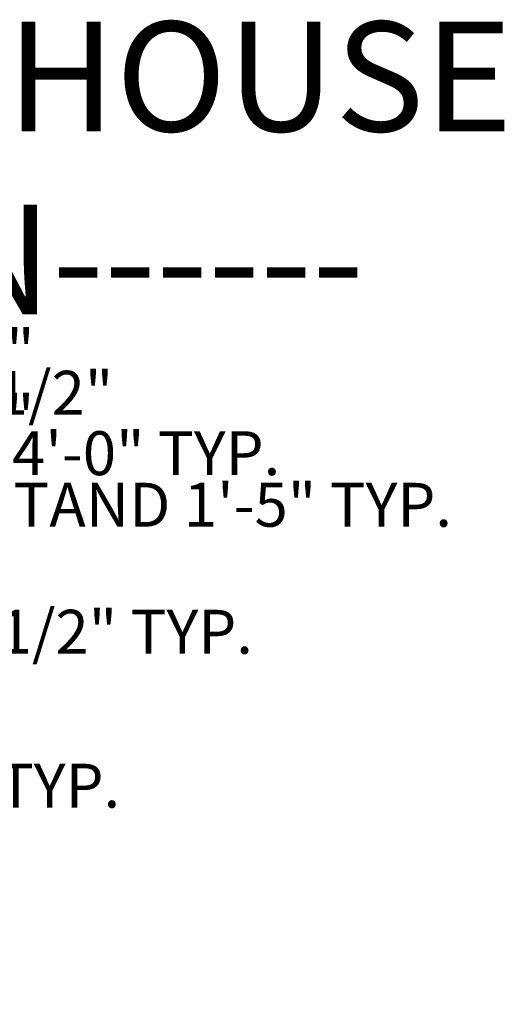
# Model space of a CAD drawing. Units: inches. Extents: x 2838 to 4029, y 1041 to 1915.
# Tile 16 of 16: x 3764 to 4029, y 1377 to 1915. Entities that reach past the tile are written whole.
import ezdxf

# ---------------------------------------------------------------- set-up
doc = ezdxf.new("R2010")
doc.units = ezdxf.units.IN
doc.header["$MEASUREMENT"] = 0
doc.layers.add('A-ANNO-DIMS', color=2, linetype='Continuous', lineweight=18)
doc.layers.add('A-ANNO-TEXT', color=7, linetype='Continuous', lineweight=18)
doc.styles.get("Standard").update_dxf_attribs({"font": 'arial.ttf'})
doc.dimstyles.get("Standard").update_dxf_attribs({"dimtxt": 24, "dimasz": 36, "dimexe": 0.18, "dimexo": 0.0625, "dimgap": 0.09, "dimtad": 0, "dimtih": 1, "dimtoh": 1, "dimdec": 0, "dimzin": 0, "dimdsep": 46, "dimlunit": 3, "dimtxsty": 'Standard', "dimcen": 0.09, "dimadec": 0, "dimazin": 0, "dimtfac": 1, "dimtdec": 0, "dimtofl": 0, "dimtmove": 0, "dimatfit": 3, "dimfxl": 1, "dimtolj": 1, "dimtzin": 0, "dimarcsym": 0})

# ---------------------------------------------------------------- blocks, each defined once
blk = doc.blocks.new('*D27')
at = {"layer": 'A-ANNO-DIMS', "color": 0, "lineweight": -2, "transparency": 16777216}
for p, q in [((3598.68, 1614.31), (3598.68, 1650.31)), ((3598.68, 1650.31), (3634.68, 1650.31)), ((3601.19, 1578.31), (3598.5, 1578.31)), ((3601.19, 1561.16), (3598.5, 1561.16)), ((3598.68, 1525.16), (3598.68, 1489.16))]:
    blk.add_line(p, q, dxfattribs=at)
at = {"layer": 'A-ANNO-DIMS', "color": 0, "transparency": 16777216}
for points in [[(3592.68, 1614.31), (3604.68, 1614.31), (3598.68, 1578.31)], [(3592.68, 1525.16), (3604.68, 1525.16), (3598.68, 1561.16)]]:
    blk.add_solid(points, dxfattribs=at)
at = {"layer": 'Defpoints', "color": 0, "transparency": 16777216}
for p in [(3598.68, 1578.31), (3601.25, 1578.31), (3601.25, 1561.16)]:
    blk.add_point(p, dxfattribs=at)
at = {"layer": 'A-ANNO-DIMS', "color": 0, "transparency": 16777216, "insert": (3820.96, 1650.31), "char_height": 24, "attachment_point": 5}
blk.add_mtext('\\A1;NIGHTSTAND 1\'-5" TYP.', dxfattribs=at)
blk = doc.blocks.new('*D28')
at = {"layer": 'A-ANNO-DIMS', "color": 0, "lineweight": -2, "transparency": 16777216}
for p, q in [((3565.25, 1580.88), (3529.25, 1580.88)), ((3601.25, 1578.37), (3601.25, 1581.06)), ((3617.82, 1578.37), (3617.82, 1581.06)), ((3653.82, 1580.88), (3689.82, 1580.88))]:
    blk.add_line(p, q, dxfattribs=at)
at = {"layer": 'A-ANNO-DIMS', "color": 0, "transparency": 16777216}
for points in [[(3565.25, 1586.88), (3565.25, 1574.88), (3601.25, 1580.88)], [(3653.82, 1586.88), (3653.82, 1574.88), (3617.82, 1580.88)]]:
    blk.add_solid(points, dxfattribs=at)
at = {"layer": 'Defpoints', "color": 0, "transparency": 16777216}
for p in [(3601.25, 1578.31), (3617.82, 1580.88), (3617.82, 1578.31)]:
    blk.add_point(p, dxfattribs=at)
at = {"layer": 'A-ANNO-DIMS', "color": 0, "transparency": 16777216, "insert": (3789.89, 1580.88), "char_height": 24, "attachment_point": 5}
blk.add_mtext('\\A1;1\'-4 1/2" TYP.', dxfattribs=at)
blk = doc.blocks.new('*D39')
at = {"layer": 'A-ANNO-DIMS', "color": 0, "lineweight": -2, "transparency": 16777216}
for p, q in [((3391.52, 1678.5), (3355.52, 1678.5)), ((3427.52, 1671.36), (3427.52, 1678.68)), ((3475.52, 1671.36), (3475.52, 1678.68)), ((3511.52, 1678.5), (3547.52, 1678.5))]:
    blk.add_line(p, q, dxfattribs=at)
at = {"layer": 'A-ANNO-DIMS', "color": 0, "transparency": 16777216}
for points in [[(3391.52, 1684.5), (3391.52, 1672.5), (3427.52, 1678.5)], [(3511.52, 1684.5), (3511.52, 1672.5), (3475.52, 1678.5)]]:
    blk.add_solid(points, dxfattribs=at)
at = {"layer": 'Defpoints', "color": 0, "transparency": 16777216}
for p in [(3475.52, 1678.5), (3427.52, 1671.3), (3475.52, 1671.3)]:
    blk.add_point(p, dxfattribs=at)
at = {"layer": 'A-ANNO-DIMS', "color": 0, "transparency": 16777216, "insert": (3732.24, 1678.5), "char_height": 24, "attachment_point": 5}
blk.add_mtext('\\A1;VENT BLOCK 4\'-0" TYP.', dxfattribs=at)
blk = doc.blocks.new('*D41')
at = {"layer": 'A-ANNO-DIMS', "color": 0, "lineweight": -2, "transparency": 16777216}
for p, q in [((3284.24, 1506.2), (3284.24, 1496.56)), ((3347.73, 1506.2), (3347.73, 1496.56)), ((3248.24, 1496.74), (3212.24, 1496.74)), ((3383.73, 1496.74), (3419.73, 1496.74))]:
    blk.add_line(p, q, dxfattribs=at)
at = {"layer": 'A-ANNO-DIMS', "color": 0, "transparency": 16777216}
for points in [[(3248.24, 1502.74), (3248.24, 1490.74), (3284.24, 1496.74)], [(3383.73, 1502.74), (3383.73, 1490.74), (3347.73, 1496.74)]]:
    blk.add_solid(points, dxfattribs=at)
at = {"layer": 'Defpoints', "color": 0, "transparency": 16777216}
for p in [(3284.24, 1506.26), (3347.73, 1506.26), (3347.73, 1496.74)]:
    blk.add_point(p, dxfattribs=at)
at = {"layer": 'A-ANNO-DIMS', "color": 0, "transparency": 16777216, "insert": (3624.81, 1496.74), "char_height": 24, "attachment_point": 5}
blk.add_mtext('\\A1;WARDROBE 5\'-3 1/2" TYP.', dxfattribs=at)
blk = doc.blocks.new('*D84')
at = {"layer": 'A-ANNO-DIMS', "color": 0, "lineweight": -2, "transparency": 16777216}
for p, q in [((3667.96, 1662.3), (3667.96, 1698.3)), ((3667.96, 1698.3), (3703.96, 1698.3)), ((3489.79, 1662.3), (3668.14, 1662.3)), ((3667.96, 1614.3), (3667.96, 1626.3)), ((3489.79, 1578.3), (3668.14, 1578.3))]:
    blk.add_line(p, q, dxfattribs=at)
at = {"layer": 'A-ANNO-DIMS', "color": 0, "transparency": 16777216}
for points in [[(3661.96, 1626.3), (3673.96, 1626.3), (3667.96, 1662.3)], [(3661.96, 1614.3), (3673.96, 1614.3), (3667.96, 1578.3)]]:
    blk.add_solid(points, dxfattribs=at)
at = {"layer": 'Defpoints', "color": 0, "transparency": 16777216}
for p in [(3489.73, 1662.3), (3667.96, 1662.3), (3489.73, 1578.3)]:
    blk.add_point(p, dxfattribs=at)
at = {"layer": 'A-ANNO-DIMS', "color": 0, "transparency": 16777216, "insert": (3735.85, 1698.3), "char_height": 24, "attachment_point": 5}
blk.add_mtext('\\A1;7\'-0"', dxfattribs=at)
blk = doc.blocks.new('*D92')
at = {"layer": 'A-ANNO-DIMS', "color": 0, "lineweight": -2, "transparency": 16777216}
for p, q in [((3585.37, 1402), (3585.37, 1081.89)), ((3618.73, 1378.66), (3618.73, 1081.89)), ((3549.37, 1082.07), (3513.37, 1082.07)), ((3654.73, 1082.07), (3690.73, 1082.07))]:
    blk.add_line(p, q, dxfattribs=at)
at = {"layer": 'A-ANNO-DIMS', "color": 0, "transparency": 16777216}
for points in [[(3549.37, 1088.07), (3549.37, 1076.07), (3585.37, 1082.07)], [(3654.73, 1088.07), (3654.73, 1076.07), (3618.73, 1082.07)]]:
    blk.add_solid(points, dxfattribs=at)
at = {"layer": 'Defpoints', "color": 0, "transparency": 16777216}
for p in [(3585.37, 1402.06), (3618.73, 1378.73), (3618.73, 1082.07)]:
    blk.add_point(p, dxfattribs=at)
at = {"layer": 'A-ANNO-DIMS', "color": 0, "transparency": 16777216, "insert": (3750.89, 1082.07), "char_height": 24, "attachment_point": 5}
blk.add_mtext('\\A1;2\'-9 1/2"', dxfattribs=at)
blk = doc.blocks.new('*D102')
at = {"layer": 'A-ANNO-DIMS', "color": 0, "lineweight": -2, "transparency": 16777216}
for p, q in [((3667.96, 1698.3), (3667.96, 1734.3)), ((3667.96, 1734.3), (3703.96, 1734.3)), ((3489.79, 1662.3), (3668.14, 1662.3)), ((3489.79, 1656.41), (3668.14, 1656.41)), ((3667.96, 1620.41), (3667.96, 1584.41))]:
    blk.add_line(p, q, dxfattribs=at)
at = {"layer": 'A-ANNO-DIMS', "color": 0, "transparency": 16777216}
for points in [[(3661.96, 1698.3), (3673.96, 1698.3), (3667.96, 1662.3)], [(3661.96, 1620.41), (3673.96, 1620.41), (3667.96, 1656.41)]]:
    blk.add_solid(points, dxfattribs=at)
at = {"layer": 'Defpoints', "color": 0, "transparency": 16777216}
for p in [(3489.73, 1662.3), (3667.96, 1662.3), (3489.73, 1656.41)]:
    blk.add_point(p, dxfattribs=at)
at = {"layer": 'A-ANNO-DIMS', "color": 0, "transparency": 16777216, "insert": (3735.95, 1734.3), "char_height": 24, "attachment_point": 5}
blk.add_mtext('\\A1;0\'-6"', dxfattribs=at)
blk = doc.blocks.new('*D105')
at = {"layer": 'A-ANNO-DIMS', "color": 0, "lineweight": -2, "transparency": 16777216}
for p, q in [((3578.46, 1711.52), (3542.46, 1711.52)), ((3614.46, 1472.42), (3614.46, 1711.7)), ((3618.73, 1469.91), (3618.73, 1711.7)), ((3654.73, 1711.52), (3690.73, 1711.52))]:
    blk.add_line(p, q, dxfattribs=at)
at = {"layer": 'A-ANNO-DIMS', "color": 0, "transparency": 16777216}
for points in [[(3578.46, 1717.52), (3578.46, 1705.52), (3614.46, 1711.52)], [(3654.73, 1717.52), (3654.73, 1705.52), (3618.73, 1711.52)]]:
    blk.add_solid(points, dxfattribs=at)
at = {"layer": 'Defpoints', "color": 0, "transparency": 16777216}
for p in [(3618.73, 1711.52), (3614.46, 1472.36), (3618.73, 1469.85)]:
    blk.add_point(p, dxfattribs=at)
at = {"layer": 'A-ANNO-DIMS', "color": 0, "transparency": 16777216, "insert": (3750.68, 1711.52), "char_height": 24, "attachment_point": 5}
blk.add_mtext('\\A1;0\'-4 1/2"', dxfattribs=at)

msp = doc.modelspace()

# ---------------------------------------------------------------- texts
at = {"layer": 'A-ANNO-TEXT', "insert": (3004.58, 1914.43), "char_height": 60, "attachment_point": 1}
msp.add_mtext_dynamic_manual_height_columns('2BHK RESIDENTIAL HOUSE \\P------2D FLOOR PLAN------', width=1981.8988, gutter_width=1, heights=[0], dxfattribs=at)

# ---------------------------------------------------------------- dimensions: what is measured, and where the dimension line sits
at = {"layer": 'A-ANNO-DIMS'}
for base, p1, p2, text, picture, middle in [((3475.52, 1678.5), (3427.52, 1671.3), (3475.52, 1671.3), 'VENT BLOCK <> TYP.', '*D39', (3732.24, 1678.5)), ((3617.82, 1580.88), (3601.25, 1578.31), (3617.82, 1578.31), '<> TYP.', '*D28', (3789.89, 1580.88)), ((3347.73, 1496.74), (3284.24, 1506.26), (3347.73, 1506.26), 'WARDROBE <> TYP.', '*D41', (3624.81, 1496.74))]:
    dim = msp.add_linear_dim(base=base, p1=p1, p2=p2, text=text, dimstyle='Standard', override={"dimdec": 1, "dimlfac": 1, "dimrnd": 0, "dimzin": 1, "dimdsep": 46, "dimlunit": 4, "dimfrac": 2}, dxfattribs=at)
    dim.commit()
    dim.dimension.update_dxf_attribs({"geometry": picture, "text_midpoint": middle})
for p1, picture, middle in [((3489.73, 1656.41), '*D102', (3735.95, 1734.3)), ((3489.73, 1578.3), '*D84', (3735.85, 1698.3))]:
    dim = msp.add_linear_dim(base=(3667.96, 1662.3), p1=p1, p2=(3489.73, 1662.3), angle=90, dimstyle='Standard', override={"dimdec": 1, "dimlfac": 1, "dimrnd": 0, "dimzin": 1, "dimdsep": 46, "dimlunit": 4, "dimfrac": 2}, dxfattribs=at)
    dim.commit()
    dim.dimension.update_dxf_attribs({"geometry": picture, "text_midpoint": middle})
for base, p1, p2, picture, middle in [((3618.73, 1711.52), (3614.46, 1472.36), (3618.73, 1469.85), '*D105', (3750.68, 1711.52)), ((3618.73, 1082.07), (3585.37, 1402.06), (3618.73, 1378.73), '*D92', (3750.89, 1082.07))]:
    dim = msp.add_linear_dim(base=base, p1=p1, p2=p2, dimstyle='Standard', override={"dimdec": 1, "dimlfac": 1, "dimrnd": 0, "dimzin": 1, "dimdsep": 46, "dimlunit": 4, "dimfrac": 2}, dxfattribs=at)
    dim.commit()
    dim.dimension.update_dxf_attribs({"geometry": picture, "text_midpoint": middle})
dim = msp.add_linear_dim(base=(3598.6826, 1578.3092), p1=(3601.2549, 1561.1604), p2=(3601.2549, 1578.3092), angle=90, text='NIGHTSTAND <> TYP.', dimstyle='Standard', override={"dimdec": 1, "dimlfac": 1, "dimrnd": 0, "dimzin": 1, "dimdsep": 46, "dimlunit": 4, "dimfrac": 2}, dxfattribs=at)
dim.commit()
dim.dimension.update_dxf_attribs({"geometry": '*D27', "text_midpoint": (3820.9609, 1650.3092)})

doc.saveas('drawing.dxf')
